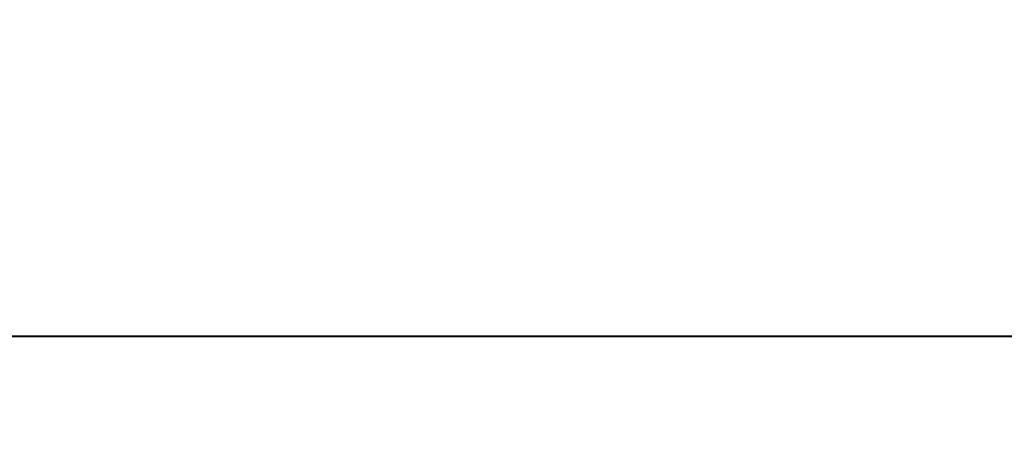
# Model space of a CAD drawing. Units: inches. Extents: x 459864 to 460310, y 324185 to 324787.
# Tile 81 of 112: x 460246.614 to 460247.1043, y 324283.4295 to 324283.6409. Entities that reach past the tile are written whole.
import ezdxf

# ---------------------------------------------------------------- set-up
doc = ezdxf.new("R2010")
doc.units = ezdxf.units.IN
for name, color, linetype, lineweight in [('A-ANNO-DIMS', 2, 'Continuous', 18), ('A-WALL', 7, 'Continuous', 40), ('L-SITE-PATT', 252, 'Continuous', 13)]:
    doc.layers.add(name, color=color, linetype=linetype, lineweight=lineweight)
doc.styles.get("Standard").update_dxf_attribs({"font": 'arial.ttf'})
doc.dimstyles.new('ISO-25', dxfattribs={"dimtxt": 6, "dimasz": 2.5, "dimexe": 1.25, "dimexo": 0.625, "dimtad": 1, "dimdec": 1, "dimlunit": 3, "dimtxsty": 'Standard', "dimcen": 2.5, "dimadec": 0, "dimazin": 0, "dimtfac": 1, "dimtdec": 1, "dimtmove": 0, "dimatfit": 3, "dimfxl": 1, "dimarcsym": 0})

# ---------------------------------------------------------------- blocks, each defined once
blk = doc.blocks.new('*D67')
at = {"layer": 'A-ANNO-DIMS', "color": 0, "lineweight": -2, "transparency": 16777216}
for p, q in [((460208.11493, 324284.10823), (460208.11493, 324315.13323)), ((460247.11493, 324284.10823), (460247.11493, 324315.13323)), ((460210.61493, 324313.88323), (460244.61493, 324313.88323))]:
    blk.add_line(p, q, dxfattribs=at)
at = {"layer": 'A-ANNO-DIMS', "color": 0, "transparency": 16777216}
for points in [[(460210.61493, 324314.2999), (460210.61493, 324313.46657), (460208.11493, 324313.88323)], [(460244.61493, 324314.2999), (460244.61493, 324313.46657), (460247.11493, 324313.88323)]]:
    blk.add_solid(points, dxfattribs=at)
at = {"layer": 'Defpoints', "color": 0, "transparency": 16777216}
for p in [(460247.11493, 324313.88323), (460208.11493, 324283.48323), (460247.11493, 324283.48323)]:
    blk.add_point(p, dxfattribs=at)
at = {"layer": 'A-ANNO-DIMS', "color": 0, "transparency": 16777216, "insert": (460227.61493, 324317.57372), "char_height": 6, "attachment_point": 5}
blk.add_mtext('3\'-3"', dxfattribs=at)

msp = doc.modelspace()

# ---------------------------------------------------------------- hatches: boundary and pattern name
at = {"layer": 'L-SITE-PATT'}
h = msp.add_hatch(dxfattribs=at)
h.set_pattern_fill('DOTS', color=256)
h.paths.add_polyline_path([(460269.80361, 324283.48323), (460247.11493, 324283.48323), (460121.92928, 324283.48323), (460121.92928, 324252.47302), (460117.42928, 324252.47302), (460110.12356, 324252.47302), (460110.12356, 324243.28654), (460080.82954, 324243.28654), (460080.82954, 324252.47302), (460061.11493, 324252.47302), (460061.11493, 324251.88242), (460077.9089, 324251.88242), (460077.9089, 324199.48323), (460080.82954, 324199.48323), (460080.82954, 324207.55322), (460110.12356, 324207.55322), (460110.12356, 324199.48323), (460110.81335, 324199.48323), (460262.11493, 324199.48323), (460269.80361, 324199.48323)], flags=17)
edge = h.paths.add_edge_path(flags=0)
edge.add_ellipse((460222.5903, 324263.81323), major_axis=(-8.48528, 8.48528), ratio=1, start_angle=405, end_angle=495, ccw=False)
edge.add_line((460214.82087, 324254.65989), (460214.83162, 324254.66592))
edge.add_ellipse((460222.5903, 324263.81323), major_axis=(-8.48528, 8.48528), ratio=1, start_angle=405, end_angle=495, ccw=False)
edge.add_line((460210.75891, 324261.78055), (460210.76758, 324261.78682))
edge.add_ellipse((460222.5903, 324263.81323), major_axis=(-8.48528, 8.48528), ratio=1, start_angle=405, end_angle=495, ccw=False)
edge.add_ellipse((460222.5903, 324263.81323), major_axis=(-8.48528, 8.48528), ratio=1, start_angle=392.754016, end_angle=405, ccw=False)
edge.add_ellipse((460222.5903, 324263.81323), major_axis=(-8.48528, 8.48528), ratio=1, start_angle=380.934718, end_angle=392.754016, ccw=False)
edge.add_line((460211.33706, 324267.98503), (460211.3404, 324267.98503))
edge.add_ellipse((460222.5903, 324263.81323), major_axis=(-8.48528, 8.48528), ratio=1, start_angle=380.934718, end_angle=392.754016, ccw=False)
edge.add_ellipse((460222.5903, 324263.81323), major_axis=(-8.48528, 8.48528), ratio=1, start_angle=347.901521, end_angle=380.934718, ccw=False)
edge.add_ellipse((460222.5903, 324263.81323), major_axis=(-8.48528, 8.48528), ratio=1, start_angle=327.061924, end_angle=347.901521, ccw=False)
edge.add_ellipse((460222.5903, 324263.81323), major_axis=(-8.48528, 8.48528), ratio=1, start_angle=278.324642, end_angle=327.061924, ccw=False)
edge.add_line((460225.15828, 324275.53599), (460225.1577, 324275.53464))
edge.add_ellipse((460222.5903, 324263.81323), major_axis=(-8.48528, 8.48528), ratio=1, start_angle=278.324642, end_angle=327.061924, ccw=False)
edge.add_ellipse((460222.5903, 324263.81323), major_axis=(-8.48528, 8.48528), ratio=1, start_angle=260.643569, end_angle=278.324642, ccw=False)
edge.add_ellipse((460222.5903, 324263.81323), major_axis=(-8.48528, 8.48528), ratio=1, start_angle=225, end_angle=260.643569, ccw=False)
edge.add_line((460234.50879, 324265.2428), (460234.50146, 324265.23944))
edge.add_ellipse((460222.5903, 324263.81323), major_axis=(-8.48528, 8.48528), ratio=1, start_angle=225, end_angle=260.643569, ccw=False)
edge.add_ellipse((460222.5903, 324263.81323), major_axis=(-8.48528, 8.48528), ratio=1, start_angle=495, end_angle=585, ccw=False)
edge.add_line((460234.43667, 324261.86121), (460234.42378, 324261.85782))
edge.add_ellipse((460222.5903, 324263.81323), major_axis=(-8.48528, 8.48528), ratio=1, start_angle=495, end_angle=585, ccw=False)
edge.add_line((460227.95013, 324253.06719), (460227.94641, 324253.08314))
edge.add_ellipse((460222.5903, 324263.81323), major_axis=(-8.48528, 8.48528), ratio=1, start_angle=495, end_angle=585, ccw=False)
edge.add_line((460226.22298, 324252.36927), (460226.21103, 324252.37955))
edge.add_ellipse((460222.5903, 324263.81323), major_axis=(-8.48528, 8.48528), ratio=1, start_angle=495, end_angle=585, ccw=False)
h.paths.add_polyline_path([(460219.65145, 324254.34665), (460218.46131, 324253.54498), (460218.27544, 324254.78932), (460219.6424, 324256.54177), (460219.62463, 324260.84756), (460216.11009, 324257.33302), (460214.34997, 324256.97807), (460215.41637, 324259.35568), (460212.52393, 324258.49582), (460213.13731, 324259.9298), (460218.50721, 324263.81323), (460222.5903, 324263.81323), (460222.5903, 324267.8067), (460218.17554, 324272.21231), (460219.02597, 324274.63898), (460222.5903, 324272.81113), (460222.5903, 324275.42332), (460223.0571, 324274.82493), (460222.67523, 324273.49221), (460225.91168, 324267.13461), (460219.62463, 324260.84756)], flags=0)
edge = h.paths.add_edge_path(flags=0)
edge.add_ellipse((460194.57576, 324264.04649), major_axis=(-8.48528, 8.48528), ratio=1, start_angle=495, end_angle=585, ccw=False)
edge.add_line((460199.93559, 324253.30046), (460199.93188, 324253.31641))
edge.add_ellipse((460194.57576, 324264.04649), major_axis=(-8.48528, 8.48528), ratio=1, start_angle=495, end_angle=585, ccw=False)
edge.add_line((460198.20844, 324252.60253), (460198.19649, 324252.61282))
edge.add_ellipse((460194.57576, 324264.04649), major_axis=(-8.48528, 8.48528), ratio=1, start_angle=495, end_angle=585, ccw=False)
edge.add_ellipse((460194.57576, 324264.04649), major_axis=(-8.48528, 8.48528), ratio=1, start_angle=405, end_angle=495, ccw=False)
edge.add_line((460186.80633, 324254.89316), (460186.81708, 324254.89919))
edge.add_ellipse((460194.57576, 324264.04649), major_axis=(-8.48528, 8.48528), ratio=1, start_angle=405, end_angle=495, ccw=False)
edge.add_line((460182.74437, 324262.01382), (460182.75305, 324262.02009))
edge.add_ellipse((460194.57576, 324264.04649), major_axis=(-8.48528, 8.48528), ratio=1, start_angle=405, end_angle=495, ccw=False)
edge.add_ellipse((460194.57576, 324264.04649), major_axis=(-8.48528, 8.48528), ratio=1, start_angle=392.754016, end_angle=405, ccw=False)
edge.add_ellipse((460194.57576, 324264.04649), major_axis=(-8.48528, 8.48528), ratio=1, start_angle=380.934718, end_angle=392.754016, ccw=False)
edge.add_line((460183.32252, 324268.21829), (460183.32587, 324268.21829))
edge.add_ellipse((460194.57576, 324264.04649), major_axis=(-8.48528, 8.48528), ratio=1, start_angle=380.934718, end_angle=392.754016, ccw=False)
edge.add_ellipse((460194.57576, 324264.04649), major_axis=(-8.48528, 8.48528), ratio=1, start_angle=347.901521, end_angle=380.934718, ccw=False)
edge.add_ellipse((460194.57576, 324264.04649), major_axis=(-8.48528, 8.48528), ratio=1, start_angle=327.061924, end_angle=347.901521, ccw=False)
edge.add_ellipse((460194.57576, 324264.04649), major_axis=(-8.48528, 8.48528), ratio=1, start_angle=278.324642, end_angle=327.061924, ccw=False)
edge.add_line((460197.14374, 324275.76926), (460197.14316, 324275.7679))
edge.add_ellipse((460194.57576, 324264.04649), major_axis=(-8.48528, 8.48528), ratio=1, start_angle=278.324642, end_angle=327.061924, ccw=False)
edge.add_ellipse((460194.57576, 324264.04649), major_axis=(-8.48528, 8.48528), ratio=1, start_angle=260.643569, end_angle=278.324642, ccw=False)
edge.add_ellipse((460194.57576, 324264.04649), major_axis=(-8.48528, 8.48528), ratio=1, start_angle=225, end_angle=260.643569, ccw=False)
edge.add_line((460206.49425, 324265.47606), (460206.48692, 324265.47271))
edge.add_ellipse((460194.57576, 324264.04649), major_axis=(-8.48528, 8.48528), ratio=1, start_angle=225, end_angle=260.643569, ccw=False)
edge.add_ellipse((460194.57576, 324264.04649), major_axis=(-8.48528, 8.48528), ratio=1, start_angle=495, end_angle=585, ccw=False)
edge.add_line((460206.42213, 324262.09448), (460206.40925, 324262.09109))
h.paths.add_polyline_path([(460191.61009, 324261.08083), (460191.63691, 324254.57992), (460190.44677, 324253.77825), (460190.2609, 324255.02259), (460191.62786, 324256.77503), (460191.61009, 324261.08083), (460188.09555, 324257.56629), (460186.33543, 324257.21133), (460187.40183, 324259.58894), (460184.5094, 324258.72909), (460185.12278, 324260.16306), (460190.49267, 324264.04649), (460194.57576, 324264.04649), (460194.57576, 324268.03996), (460190.161, 324272.44558), (460191.01143, 324274.87225), (460194.57576, 324273.04439), (460194.57576, 324275.65659), (460195.04256, 324275.0582), (460194.66069, 324273.72548), (460197.89714, 324267.36788)], flags=0)
edge = h.paths.add_edge_path(flags=0)
edge.add_ellipse((460252.91196, 324263.57762), major_axis=(-8.48528, 8.48528), ratio=1, start_angle=405, end_angle=495, ccw=False)
edge.add_line((460241.08058, 324261.54494), (460241.08925, 324261.55121))
edge.add_ellipse((460252.91196, 324263.57762), major_axis=(-8.48528, 8.48528), ratio=1, start_angle=405, end_angle=495, ccw=False)
edge.add_ellipse((460252.91196, 324263.57762), major_axis=(-8.48528, 8.48528), ratio=1, start_angle=392.754016, end_angle=405, ccw=False)
edge.add_ellipse((460252.91196, 324263.57762), major_axis=(-8.48528, 8.48528), ratio=1, start_angle=380.934718, end_angle=392.754016, ccw=False)
edge.add_line((460241.65872, 324267.74942), (460241.66207, 324267.74942))
edge.add_ellipse((460252.91196, 324263.57762), major_axis=(-8.48528, 8.48528), ratio=1, start_angle=380.934718, end_angle=392.754016, ccw=False)
edge.add_ellipse((460252.91196, 324263.57762), major_axis=(-8.48528, 8.48528), ratio=1, start_angle=347.901521, end_angle=380.934718, ccw=False)
edge.add_ellipse((460252.91196, 324263.57762), major_axis=(-8.48528, 8.48528), ratio=1, start_angle=327.061924, end_angle=347.901521, ccw=False)
edge.add_ellipse((460252.91196, 324263.57762), major_axis=(-8.48528, 8.48528), ratio=1, start_angle=278.324642, end_angle=327.061924, ccw=False)
edge.add_line((460255.47994, 324275.30038), (460255.47936, 324275.29902))
edge.add_ellipse((460252.91196, 324263.57762), major_axis=(-8.48528, 8.48528), ratio=1, start_angle=278.324642, end_angle=327.061924, ccw=False)
edge.add_ellipse((460252.91196, 324263.57762), major_axis=(-8.48528, 8.48528), ratio=1, start_angle=260.643569, end_angle=278.324642, ccw=False)
edge.add_ellipse((460252.91196, 324263.57762), major_axis=(-8.48528, 8.48528), ratio=1, start_angle=225, end_angle=260.643569, ccw=False)
edge.add_line((460264.83046, 324265.00718), (460264.82312, 324265.00383))
edge.add_ellipse((460252.91196, 324263.57762), major_axis=(-8.48528, 8.48528), ratio=1, start_angle=225, end_angle=260.643569, ccw=False)
edge.add_ellipse((460252.91196, 324263.57762), major_axis=(-8.48528, 8.48528), ratio=1, start_angle=495, end_angle=585, ccw=False)
edge.add_line((460264.75833, 324261.6256), (460264.74545, 324261.62221))
edge.add_ellipse((460252.91196, 324263.57762), major_axis=(-8.48528, 8.48528), ratio=1, start_angle=495, end_angle=585, ccw=False)
edge.add_line((460258.2718, 324252.83158), (460258.26808, 324252.84753))
edge.add_ellipse((460252.91196, 324263.57762), major_axis=(-8.48528, 8.48528), ratio=1, start_angle=495, end_angle=585, ccw=False)
edge.add_line((460256.54464, 324252.13365), (460256.5327, 324252.14394))
edge.add_ellipse((460252.91196, 324263.57762), major_axis=(-8.48528, 8.48528), ratio=1, start_angle=495, end_angle=585, ccw=False)
edge.add_ellipse((460252.91196, 324263.57762), major_axis=(-8.48528, 8.48528), ratio=1, start_angle=405, end_angle=495, ccw=False)
edge.add_line((460245.14253, 324254.42428), (460245.15329, 324254.43031))
h.paths.add_polyline_path([(460244.67163, 324256.74245), (460245.73803, 324259.12007), (460242.8456, 324258.26021), (460243.45898, 324259.69418), (460248.82888, 324263.57762), (460252.91196, 324263.57762), (460252.91196, 324267.57108), (460248.4972, 324271.9767), (460249.34763, 324274.40337), (460252.91196, 324272.57552), (460252.91196, 324275.18771), (460253.37876, 324274.58932), (460252.9969, 324273.2566), (460256.23334, 324266.899), (460249.9463, 324260.61195), (460249.97312, 324254.11104), (460248.78298, 324253.30937), (460248.5971, 324254.55371), (460249.96406, 324256.30615), (460249.9463, 324260.61195), (460246.43175, 324257.09741)], flags=0)
edge = h.paths.add_edge_path(flags=0)
edge.add_ellipse((460167.43869, 324262.83279), major_axis=(-8.48528, 8.48528), ratio=1, start_angle=495, end_angle=585, ccw=False)
edge.add_line((460172.79852, 324252.08676), (460172.79481, 324252.1027))
edge.add_ellipse((460167.43869, 324262.83279), major_axis=(-8.48528, 8.48528), ratio=1, start_angle=495, end_angle=585, ccw=False)
edge.add_line((460171.07137, 324251.38883), (460171.05942, 324251.39911))
edge.add_ellipse((460167.43869, 324262.83279), major_axis=(-8.48528, 8.48528), ratio=1, start_angle=495, end_angle=585, ccw=False)
edge.add_ellipse((460167.43869, 324262.83279), major_axis=(-8.48528, 8.48528), ratio=1, start_angle=405, end_angle=495, ccw=False)
edge.add_line((460159.66926, 324253.67945), (460159.68001, 324253.68548))
edge.add_ellipse((460167.43869, 324262.83279), major_axis=(-8.48528, 8.48528), ratio=1, start_angle=405, end_angle=495, ccw=False)
edge.add_line((460155.6073, 324260.80011), (460155.61598, 324260.80639))
edge.add_ellipse((460167.43869, 324262.83279), major_axis=(-8.48528, 8.48528), ratio=1, start_angle=405, end_angle=495, ccw=False)
edge.add_ellipse((460167.43869, 324262.83279), major_axis=(-8.48528, 8.48528), ratio=1, start_angle=392.754016, end_angle=405, ccw=False)
edge.add_ellipse((460167.43869, 324262.83279), major_axis=(-8.48528, 8.48528), ratio=1, start_angle=380.934718, end_angle=392.754016, ccw=False)
edge.add_line((460156.18545, 324267.00459), (460156.1888, 324267.00459))
edge.add_ellipse((460167.43869, 324262.83279), major_axis=(-8.48528, 8.48528), ratio=1, start_angle=380.934718, end_angle=392.754016, ccw=False)
edge.add_ellipse((460167.43869, 324262.83279), major_axis=(-8.48528, 8.48528), ratio=1, start_angle=347.901521, end_angle=380.934718, ccw=False)
edge.add_ellipse((460167.43869, 324262.83279), major_axis=(-8.48528, 8.48528), ratio=1, start_angle=327.061924, end_angle=347.901521, ccw=False)
edge.add_ellipse((460167.43869, 324262.83279), major_axis=(-8.48528, 8.48528), ratio=1, start_angle=278.324642, end_angle=327.061924, ccw=False)
edge.add_line((460170.00667, 324274.55555), (460170.00609, 324274.5542))
edge.add_ellipse((460167.43869, 324262.83279), major_axis=(-8.48528, 8.48528), ratio=1, start_angle=278.324642, end_angle=327.061924, ccw=False)
edge.add_ellipse((460167.43869, 324262.83279), major_axis=(-8.48528, 8.48528), ratio=1, start_angle=260.643569, end_angle=278.324642, ccw=False)
edge.add_ellipse((460167.43869, 324262.83279), major_axis=(-8.48528, 8.48528), ratio=1, start_angle=225, end_angle=260.643569, ccw=False)
edge.add_line((460179.35719, 324264.26236), (460179.34985, 324264.259))
edge.add_ellipse((460167.43869, 324262.83279), major_axis=(-8.48528, 8.48528), ratio=1, start_angle=225, end_angle=260.643569, ccw=False)
edge.add_ellipse((460167.43869, 324262.83279), major_axis=(-8.48528, 8.48528), ratio=1, start_angle=495, end_angle=585, ccw=False)
edge.add_line((460179.28506, 324260.88078), (460179.27218, 324260.87738))
h.paths.add_polyline_path([(460164.47302, 324259.86713), (460164.49985, 324253.36622), (460163.30971, 324252.56455), (460163.12383, 324253.80888), (460164.49079, 324255.56133), (460164.47302, 324259.86713), (460160.95848, 324256.35258), (460159.19836, 324255.99763), (460160.26476, 324258.37524), (460157.37233, 324257.51539), (460157.98571, 324258.94936), (460163.35561, 324262.83279), (460167.43869, 324262.83279), (460167.43869, 324266.82626), (460163.02393, 324271.23187), (460163.87436, 324273.65854), (460167.43869, 324271.83069), (460167.43869, 324274.44288), (460167.90549, 324273.84449), (460167.52362, 324272.51177), (460170.76007, 324266.15417)], flags=0)
edge = h.paths.add_edge_path(flags=0)
edge.add_ellipse((460140.75809, 324262.36958), major_axis=(-8.48528, 8.48528), ratio=1, start_angle=495, end_angle=585, ccw=False)
edge.add_line((460146.11792, 324251.62355), (460146.11421, 324251.6395))
edge.add_ellipse((460140.75809, 324262.36958), major_axis=(-8.48528, 8.48528), ratio=1, start_angle=495, end_angle=585, ccw=False)
edge.add_line((460144.39077, 324250.92562), (460144.37882, 324250.93591))
edge.add_ellipse((460140.75809, 324262.36958), major_axis=(-8.48528, 8.48528), ratio=1, start_angle=495, end_angle=585, ccw=False)
edge.add_ellipse((460140.75809, 324262.36958), major_axis=(-8.48528, 8.48528), ratio=1, start_angle=405, end_angle=495, ccw=False)
edge.add_line((460132.98866, 324253.21625), (460132.99941, 324253.22228))
edge.add_ellipse((460140.75809, 324262.36958), major_axis=(-8.48528, 8.48528), ratio=1, start_angle=405, end_angle=495, ccw=False)
edge.add_line((460128.9267, 324260.33691), (460128.93538, 324260.34318))
edge.add_ellipse((460140.75809, 324262.36958), major_axis=(-8.48528, 8.48528), ratio=1, start_angle=405, end_angle=495, ccw=False)
edge.add_ellipse((460140.75809, 324262.36958), major_axis=(-8.48528, 8.48528), ratio=1, start_angle=392.754016, end_angle=405, ccw=False)
edge.add_ellipse((460140.75809, 324262.36958), major_axis=(-8.48528, 8.48528), ratio=1, start_angle=380.934718, end_angle=392.754016, ccw=False)
edge.add_line((460129.50485, 324266.54138), (460129.5082, 324266.54138))
edge.add_ellipse((460140.75809, 324262.36958), major_axis=(-8.48528, 8.48528), ratio=1, start_angle=380.934718, end_angle=392.754016, ccw=False)
edge.add_ellipse((460140.75809, 324262.36958), major_axis=(-8.48528, 8.48528), ratio=1, start_angle=347.901521, end_angle=380.934718, ccw=False)
edge.add_ellipse((460140.75809, 324262.36958), major_axis=(-8.48528, 8.48528), ratio=1, start_angle=327.061924, end_angle=347.901521, ccw=False)
edge.add_ellipse((460140.75809, 324262.36958), major_axis=(-8.48528, 8.48528), ratio=1, start_angle=278.324642, end_angle=327.061924, ccw=False)
edge.add_line((460143.32607, 324274.09235), (460143.32549, 324274.09099))
edge.add_ellipse((460140.75809, 324262.36958), major_axis=(-8.48528, 8.48528), ratio=1, start_angle=278.324642, end_angle=327.061924, ccw=False)
edge.add_ellipse((460140.75809, 324262.36958), major_axis=(-8.48528, 8.48528), ratio=1, start_angle=260.643569, end_angle=278.324642, ccw=False)
edge.add_ellipse((460140.75809, 324262.36958), major_axis=(-8.48528, 8.48528), ratio=1, start_angle=225, end_angle=260.643569, ccw=False)
edge.add_line((460152.67658, 324263.79915), (460152.66925, 324263.7958))
edge.add_ellipse((460140.75809, 324262.36958), major_axis=(-8.48528, 8.48528), ratio=1, start_angle=225, end_angle=260.643569, ccw=False)
edge.add_ellipse((460140.75809, 324262.36958), major_axis=(-8.48528, 8.48528), ratio=1, start_angle=495, end_angle=585, ccw=False)
edge.add_line((460152.60446, 324260.41757), (460152.59158, 324260.41418))
h.paths.add_polyline_path([(460137.79242, 324259.40392), (460137.81925, 324252.90301), (460136.6291, 324252.10134), (460136.44323, 324253.34568), (460137.81019, 324255.09812), (460137.79242, 324259.40392), (460134.27788, 324255.88938), (460132.51776, 324255.53442), (460133.58416, 324257.91203), (460130.69173, 324257.05218), (460131.30511, 324258.48615), (460136.675, 324262.36958), (460140.75809, 324262.36958), (460140.75809, 324266.36305), (460136.34333, 324270.76867), (460137.19376, 324273.19534), (460140.75809, 324271.36749), (460140.75809, 324273.97968), (460141.22489, 324273.38129), (460140.84302, 324272.04857), (460144.07947, 324265.69097)], flags=0)
h.paths.add_polyline_path([(460110.12356, 324227.41387), (460080.82954, 324227.41387), (460080.82954, 324235.48385), (460110.12356, 324235.48385)], flags=16)
h.paths.add_polyline_path([(460110.12356, 324220.79663), (460110.12356, 324212.72665), (460080.82954, 324212.72665), (460080.82954, 324220.79663)], flags=16)
h.paths.add_polyline_path([(460269.80361, 324283.48323), (460247.11493, 324283.48323), (460121.92928, 324283.48323), (460121.92928, 324252.47302), (460117.42928, 324252.47302), (460110.12356, 324252.47302), (460110.12356, 324243.28654), (460080.82954, 324243.28654), (460080.82954, 324252.47302), (460061.11493, 324252.47302), (460061.11493, 324251.88242), (460077.9089, 324251.88242), (460077.9089, 324199.48323), (460080.82954, 324199.48323), (460080.82954, 324207.55322), (460110.12356, 324207.55322), (460110.12356, 324199.48323), (460262.11493, 324199.48323), (460269.80361, 324199.48323)], flags=17)
h.paths.add_polyline_path([(460219.65145, 324254.34665), (460218.46131, 324253.54498), (460218.27544, 324254.78932), (460219.6424, 324256.54177), (460219.62463, 324260.84756), (460216.11009, 324257.33302), (460214.34997, 324256.97807), (460215.41637, 324259.35568), (460212.52393, 324258.49582), (460213.13731, 324259.9298), (460218.50721, 324263.81323), (460222.5903, 324263.81323), (460220.18049, 324266.22304), (460215.46096, 324265.30765), (460211.83453, 324266.13655), (460216.24662, 324267.98503), (460218.4185, 324267.98503), (460222.5903, 324263.81323), (460222.5903, 324267.8067), (460218.17554, 324272.21231), (460219.02597, 324274.63898), (460222.5903, 324272.81113), (460222.5903, 324275.42332), (460223.0571, 324274.82493), (460222.67523, 324273.49221), (460225.91168, 324267.13461), (460222.5903, 324263.81323), (460231.38287, 324263.81323), (460228.48472, 324262.48783), (460224.42521, 324261.97832), (460228.6799, 324257.72362), (460228.96584, 324254.79101), (460227.14177, 324256.53663), (460227.54207, 324254.81857), (460227.33334, 324253.61447), (460222.5903, 324259.98463), (460222.5903, 324255.49667), (460221.37741, 324256.54085), (460220.57579, 324261.79873), (460219.62463, 324260.84756)], flags=0)
h.paths.add_polyline_path([(460199.12723, 324256.7699), (460199.52753, 324255.05184), (460199.31881, 324253.84773), (460194.57576, 324260.21789), (460194.57576, 324255.72993), (460193.36287, 324256.77411), (460192.56126, 324262.03199), (460191.61009, 324261.08083), (460191.63691, 324254.57992), (460190.44677, 324253.77825), (460190.2609, 324255.02259), (460191.62786, 324256.77503), (460191.61009, 324261.08083), (460188.09555, 324257.56629), (460186.33543, 324257.21133), (460187.40183, 324259.58894), (460184.5094, 324258.72909), (460185.12278, 324260.16306), (460190.49267, 324264.04649), (460194.57576, 324264.04649), (460192.16595, 324266.4563), (460187.44642, 324265.54091), (460183.82, 324266.36982), (460188.23208, 324268.21829), (460190.40396, 324268.21829), (460194.57576, 324264.04649), (460194.57576, 324268.03996), (460190.161, 324272.44558), (460191.01143, 324274.87225), (460194.57576, 324273.04439), (460194.57576, 324275.65659), (460195.04256, 324275.0582), (460194.66069, 324273.72548), (460197.89714, 324267.36788), (460194.57576, 324264.04649), (460203.36833, 324264.04649), (460200.47018, 324262.72109), (460196.41067, 324262.21158), (460200.66536, 324257.95689), (460200.9513, 324255.02428)], flags=0)
h.paths.add_polyline_path([(460244.67163, 324256.74245), (460245.73803, 324259.12007), (460242.8456, 324258.26021), (460243.45898, 324259.69418), (460248.82888, 324263.57762), (460252.91196, 324263.57762), (460250.50215, 324265.98742), (460245.78262, 324265.07203), (460242.1562, 324265.90094), (460246.56828, 324267.74942), (460248.74016, 324267.74942), (460252.91196, 324263.57762), (460252.91196, 324267.57108), (460248.4972, 324271.9767), (460249.34763, 324274.40337), (460252.91196, 324272.57552), (460252.91196, 324275.18771), (460253.37876, 324274.58932), (460252.9969, 324273.2566), (460256.23334, 324266.899), (460252.91196, 324263.57762), (460261.70454, 324263.57762), (460258.80638, 324262.25221), (460254.74687, 324261.7427), (460259.00157, 324257.48801), (460259.2875, 324254.5554), (460257.46343, 324256.30102), (460257.86373, 324254.58296), (460257.65501, 324253.37885), (460252.91196, 324259.74901), (460252.91196, 324255.26105), (460251.69907, 324256.30524), (460250.89746, 324261.56311), (460249.9463, 324260.61195), (460249.97312, 324254.11104), (460248.78298, 324253.30937), (460248.5971, 324254.55371), (460249.96406, 324256.30615), (460249.9463, 324260.61195), (460246.43175, 324257.09741)], flags=0)
h.paths.add_polyline_path([(460173.52829, 324256.74319), (460173.81423, 324253.81058), (460171.99016, 324255.55619), (460172.39046, 324253.83814), (460172.18174, 324252.63403), (460167.43869, 324259.00419), (460167.43869, 324254.51623), (460166.2258, 324255.56041), (460165.42419, 324260.81829), (460164.47302, 324259.86713), (460164.49985, 324253.36622), (460163.30971, 324252.56455), (460163.12383, 324253.80888), (460164.49079, 324255.56133), (460164.47302, 324259.86713), (460160.95848, 324256.35258), (460159.19836, 324255.99763), (460160.26476, 324258.37524), (460157.37233, 324257.51539), (460157.98571, 324258.94936), (460163.35561, 324262.83279), (460167.43869, 324262.83279), (460165.02888, 324265.2426), (460160.30935, 324264.32721), (460156.68293, 324265.15611), (460161.09501, 324267.00459), (460163.26689, 324267.00459), (460167.43869, 324262.83279), (460167.43869, 324266.82626), (460163.02393, 324271.23187), (460163.87436, 324273.65854), (460167.43869, 324271.83069), (460167.43869, 324274.44288), (460167.90549, 324273.84449), (460167.52362, 324272.51177), (460170.76007, 324266.15417), (460167.43869, 324262.83279), (460176.23127, 324262.83279), (460173.33311, 324261.50739), (460169.2736, 324260.99788)], flags=0)
h.paths.add_polyline_path([(460146.84769, 324256.27998), (460147.13363, 324253.34737), (460145.30956, 324255.09299), (460145.70986, 324253.37493), (460145.50114, 324252.17082), (460140.75809, 324258.54098), (460140.75809, 324254.05302), (460139.5452, 324255.0972), (460138.74359, 324260.35508), (460137.79242, 324259.40392), (460137.81925, 324252.90301), (460136.6291, 324252.10134), (460136.44323, 324253.34568), (460137.81019, 324255.09812), (460137.79242, 324259.40392), (460134.27788, 324255.88938), (460132.51776, 324255.53442), (460133.58416, 324257.91203), (460130.69173, 324257.05218), (460131.30511, 324258.48615), (460136.675, 324262.36958), (460140.75809, 324262.36958), (460138.34828, 324264.77939), (460133.62875, 324263.864), (460130.00233, 324264.69291), (460134.41441, 324266.54138), (460136.58629, 324266.54138), (460140.75809, 324262.36958), (460140.75809, 324266.36305), (460136.34333, 324270.76867), (460137.19376, 324273.19534), (460140.75809, 324271.36749), (460140.75809, 324273.97968), (460141.22489, 324273.38129), (460140.84302, 324272.04857), (460144.07947, 324265.69097), (460140.75809, 324262.36958), (460149.55066, 324262.36958), (460146.65251, 324261.04418), (460142.593, 324260.53467)], flags=0)
edge = h.paths.add_edge_path()
edge.add_line((460269.80361, 324272.54905), (460260.88148, 324272.54905))
edge.add_ellipse((460252.91196, 324263.57762), major_axis=(-8.48528, 8.48528), ratio=1, start_angle=260.643569, end_angle=273.384624, ccw=False)
edge.add_line((460262.28261, 324271.09211), (460262.26055, 324271.09106))
edge.add_ellipse((460252.91196, 324263.57762), major_axis=(-8.48528, 8.48528), ratio=1, start_angle=260.643569, end_angle=273.384624, ccw=False)
edge.add_ellipse((460252.91196, 324263.57762), major_axis=(-8.48528, 8.48528), ratio=1, start_angle=225, end_angle=260.643569, ccw=False)
edge.add_line((460263.60857, 324269.06329), (460263.57165, 324269.05828))
edge.add_ellipse((460252.91196, 324263.57762), major_axis=(-8.48528, 8.48528), ratio=1, start_angle=225, end_angle=260.643569, ccw=False)
edge.add_line((460264.61546, 324266.30554), (460264.58536, 324266.3052))
edge.add_ellipse((460252.91196, 324263.57762), major_axis=(-8.48528, 8.48528), ratio=1, start_angle=225, end_angle=260.643569, ccw=False)
edge.add_line((460264.83046, 324265.00718), (460264.82312, 324265.00383))
edge.add_ellipse((460252.91196, 324263.57762), major_axis=(-8.48528, 8.48528), ratio=1, start_angle=225, end_angle=260.643569, ccw=False)
edge.add_ellipse((460252.91196, 324263.57762), major_axis=(-8.48528, 8.48528), ratio=1, start_angle=495, end_angle=585, ccw=False)
edge.add_line((460264.75833, 324261.6256), (460264.74545, 324261.62221))
edge.add_ellipse((460252.91196, 324263.57762), major_axis=(-8.48528, 8.48528), ratio=1, start_angle=495, end_angle=585, ccw=False)
edge.add_line((460263.4422, 324257.73902), (460263.38926, 324257.77924))
edge.add_ellipse((460252.91196, 324263.57762), major_axis=(-8.48528, 8.48528), ratio=1, start_angle=495, end_angle=585, ccw=False)
edge.add_line((460258.12807, 324252.7435), (460258.10188, 324252.77868))
edge.add_ellipse((460252.91196, 324263.57762), major_axis=(-8.48528, 8.48528), ratio=1, start_angle=495, end_angle=585, ccw=False)
edge.add_line((460256.54464, 324252.13365), (460256.5327, 324252.14394))
edge.add_ellipse((460252.91196, 324263.57762), major_axis=(-8.48528, 8.48528), ratio=1, start_angle=495, end_angle=585, ccw=False)
edge.add_ellipse((460252.91196, 324263.57762), major_axis=(-8.48528, 8.48528), ratio=1, start_angle=405, end_angle=495, ccw=False)
edge.add_line((460250.59399, 324251.78041), (460250.60465, 324251.81982))
edge.add_ellipse((460252.91196, 324263.57762), major_axis=(-8.48528, 8.48528), ratio=1, start_angle=405, end_angle=495, ccw=False)
edge.add_line((460245.14253, 324254.42428), (460245.15329, 324254.43031))
edge.add_ellipse((460252.91196, 324263.57762), major_axis=(-8.48528, 8.48528), ratio=1, start_angle=405, end_angle=495, ccw=False)
edge.add_line((460243.52459, 324256.059), (460243.56034, 324256.09136))
edge.add_ellipse((460252.91196, 324263.57762), major_axis=(-8.48528, 8.48528), ratio=1, start_angle=405, end_angle=495, ccw=False)
edge.add_line((460241.4401, 324259.89273), (460241.52244, 324259.89588))
edge.add_ellipse((460252.91196, 324263.57762), major_axis=(-8.48528, 8.48528), ratio=1, start_angle=405, end_angle=495, ccw=False)
edge.add_line((460241.08058, 324261.54494), (460241.08925, 324261.55121))
edge.add_ellipse((460252.91196, 324263.57762), major_axis=(-8.48528, 8.48528), ratio=1, start_angle=405, end_angle=495, ccw=False)
edge.add_ellipse((460252.91196, 324263.57762), major_axis=(-8.48528, 8.48528), ratio=1, start_angle=392.754016, end_angle=405, ccw=False)
edge.add_line((460241.0503, 324265.43761), (460241.06257, 324265.44275))
edge.add_ellipse((460252.91196, 324263.57762), major_axis=(-8.48528, 8.48528), ratio=1, start_angle=392.754016, end_angle=405, ccw=False)
edge.add_ellipse((460252.91196, 324263.57762), major_axis=(-8.48528, 8.48528), ratio=1, start_angle=380.934718, end_angle=392.754016, ccw=False)
edge.add_line((460241.45189, 324267.17639), (460241.46904, 324267.17099))
edge.add_ellipse((460252.91196, 324263.57762), major_axis=(-8.48528, 8.48528), ratio=1, start_angle=380.934718, end_angle=392.754016, ccw=False)
edge.add_line((460241.65872, 324267.74942), (460241.66207, 324267.74942))
edge.add_ellipse((460252.91196, 324263.57762), major_axis=(-8.48528, 8.48528), ratio=1, start_angle=380.934718, end_angle=392.754016, ccw=False)
edge.add_ellipse((460252.91196, 324263.57762), major_axis=(-8.48528, 8.48528), ratio=1, start_angle=356.615376, end_angle=380.934718, ccw=False)
edge.add_line((460244.88029, 324272.48765), (460244.71265, 324272.54905))
edge.add_line((460244.71265, 324272.54905), (460230.81741, 324272.54905))
edge.add_ellipse((460222.5903, 324263.81323), major_axis=(-8.48528, 8.48528), ratio=1, start_angle=260.643569, end_angle=271.717775, ccw=False)
edge.add_ellipse((460222.5903, 324263.81323), major_axis=(-8.48528, 8.48528), ratio=1, start_angle=225, end_angle=260.643569, ccw=False)
edge.add_line((460233.2869, 324269.29891), (460233.24999, 324269.2939))
edge.add_ellipse((460222.5903, 324263.81323), major_axis=(-8.48528, 8.48528), ratio=1, start_angle=225, end_angle=260.643569, ccw=False)
edge.add_line((460234.2938, 324266.54115), (460234.26369, 324266.54081))
edge.add_ellipse((460222.5903, 324263.81323), major_axis=(-8.48528, 8.48528), ratio=1, start_angle=225, end_angle=260.643569, ccw=False)
edge.add_line((460234.50879, 324265.2428), (460234.50146, 324265.23944))
edge.add_ellipse((460222.5903, 324263.81323), major_axis=(-8.48528, 8.48528), ratio=1, start_angle=225, end_angle=260.643569, ccw=False)
edge.add_ellipse((460222.5903, 324263.81323), major_axis=(-8.48528, 8.48528), ratio=1, start_angle=495, end_angle=585, ccw=False)
edge.add_line((460234.43667, 324261.86121), (460234.42378, 324261.85782))
edge.add_ellipse((460222.5903, 324263.81323), major_axis=(-8.48528, 8.48528), ratio=1, start_angle=495, end_angle=585, ccw=False)
edge.add_line((460233.12054, 324257.97463), (460233.06759, 324258.01485))
edge.add_ellipse((460222.5903, 324263.81323), major_axis=(-8.48528, 8.48528), ratio=1, start_angle=495, end_angle=585, ccw=False)
edge.add_line((460227.8064, 324252.97912), (460227.78021, 324253.0143))
edge.add_ellipse((460222.5903, 324263.81323), major_axis=(-8.48528, 8.48528), ratio=1, start_angle=495, end_angle=585, ccw=False)
edge.add_line((460226.22298, 324252.36927), (460226.21103, 324252.37955))
edge.add_ellipse((460222.5903, 324263.81323), major_axis=(-8.48528, 8.48528), ratio=1, start_angle=495, end_angle=585, ccw=False)
edge.add_ellipse((460222.5903, 324263.81323), major_axis=(-8.48528, 8.48528), ratio=1, start_angle=405, end_angle=495, ccw=False)
edge.add_line((460220.27232, 324252.01602), (460220.28299, 324252.05543))
edge.add_ellipse((460222.5903, 324263.81323), major_axis=(-8.48528, 8.48528), ratio=1, start_angle=405, end_angle=495, ccw=False)
edge.add_line((460214.82087, 324254.65989), (460214.83162, 324254.66592))
edge.add_ellipse((460222.5903, 324263.81323), major_axis=(-8.48528, 8.48528), ratio=1, start_angle=405, end_angle=495, ccw=False)
edge.add_line((460213.20292, 324256.29462), (460213.23868, 324256.32697))
edge.add_ellipse((460222.5903, 324263.81323), major_axis=(-8.48528, 8.48528), ratio=1, start_angle=405, end_angle=495, ccw=False)
edge.add_line((460211.11844, 324260.12834), (460211.20077, 324260.13149))
edge.add_ellipse((460222.5903, 324263.81323), major_axis=(-8.48528, 8.48528), ratio=1, start_angle=405, end_angle=495, ccw=False)
edge.add_line((460210.75891, 324261.78055), (460210.76758, 324261.78682))
edge.add_ellipse((460222.5903, 324263.81323), major_axis=(-8.48528, 8.48528), ratio=1, start_angle=405, end_angle=495, ccw=False)
edge.add_ellipse((460222.5903, 324263.81323), major_axis=(-8.48528, 8.48528), ratio=1, start_angle=392.754016, end_angle=405, ccw=False)
edge.add_line((460210.72863, 324265.67323), (460210.7409, 324265.67836))
edge.add_ellipse((460222.5903, 324263.81323), major_axis=(-8.48528, 8.48528), ratio=1, start_angle=392.754016, end_angle=405, ccw=False)
edge.add_ellipse((460222.5903, 324263.81323), major_axis=(-8.48528, 8.48528), ratio=1, start_angle=380.934718, end_angle=392.754016, ccw=False)
edge.add_line((460211.13022, 324267.412), (460211.14738, 324267.4066))
edge.add_ellipse((460222.5903, 324263.81323), major_axis=(-8.48528, 8.48528), ratio=1, start_angle=380.934718, end_angle=392.754016, ccw=False)
edge.add_line((460211.33706, 324267.98503), (460211.3404, 324267.98503))
edge.add_ellipse((460222.5903, 324263.81323), major_axis=(-8.48528, 8.48528), ratio=1, start_angle=380.934718, end_angle=392.754016, ccw=False)
edge.add_ellipse((460222.5903, 324263.81323), major_axis=(-8.48528, 8.48528), ratio=1, start_angle=358.282225, end_angle=380.934718, ccw=False)
edge.add_line((460213.70452, 324271.90183), (460213.70904, 324271.86897))
edge.add_ellipse((460222.5903, 324263.81323), major_axis=(-8.48528, 8.48528), ratio=1, start_angle=358.282225, end_angle=380.934718, ccw=False)
edge.add_line((460214.36318, 324272.54905), (460203.07832, 324272.54905))
edge.add_line((460203.07832, 324272.54905), (460203.06034, 324272.53108))
edge.add_ellipse((460194.57576, 324264.04649), major_axis=(-8.48528, 8.48528), ratio=1, start_angle=260.643569, end_angle=270.11679, ccw=False)
edge.add_line((460203.95659, 324271.56147), (460203.92091, 324271.55978))
edge.add_ellipse((460194.57576, 324264.04649), major_axis=(-8.48528, 8.48528), ratio=1, start_angle=260.643569, end_angle=270.11679, ccw=False)
edge.add_ellipse((460194.57576, 324264.04649), major_axis=(-8.48528, 8.48528), ratio=1, start_angle=225, end_angle=260.643569, ccw=False)
edge.add_line((460205.27237, 324269.53217), (460205.23545, 324269.52716))
edge.add_ellipse((460194.57576, 324264.04649), major_axis=(-8.48528, 8.48528), ratio=1, start_angle=225, end_angle=260.643569, ccw=False)
edge.add_line((460206.27926, 324266.77442), (460206.24915, 324266.77407))
edge.add_ellipse((460194.57576, 324264.04649), major_axis=(-8.48528, 8.48528), ratio=1, start_angle=225, end_angle=260.643569, ccw=False)
edge.add_line((460206.49425, 324265.47606), (460206.48692, 324265.47271))
edge.add_ellipse((460194.57576, 324264.04649), major_axis=(-8.48528, 8.48528), ratio=1, start_angle=225, end_angle=260.643569, ccw=False)
edge.add_ellipse((460194.57576, 324264.04649), major_axis=(-8.48528, 8.48528), ratio=1, start_angle=495, end_angle=585, ccw=False)
edge.add_line((460206.42213, 324262.09448), (460206.40925, 324262.09109))
edge.add_ellipse((460194.57576, 324264.04649), major_axis=(-8.48528, 8.48528), ratio=1, start_angle=495, end_angle=585, ccw=False)
edge.add_line((460205.106, 324258.2079), (460205.05306, 324258.24812))
edge.add_ellipse((460194.57576, 324264.04649), major_axis=(-8.48528, 8.48528), ratio=1, start_angle=495, end_angle=585, ccw=False)
edge.add_line((460199.79187, 324253.21238), (460199.76568, 324253.24756))
edge.add_ellipse((460194.57576, 324264.04649), major_axis=(-8.48528, 8.48528), ratio=1, start_angle=495, end_angle=585, ccw=False)
edge.add_line((460198.20844, 324252.60253), (460198.19649, 324252.61282))
edge.add_ellipse((460194.57576, 324264.04649), major_axis=(-8.48528, 8.48528), ratio=1, start_angle=495, end_angle=585, ccw=False)
edge.add_ellipse((460194.57576, 324264.04649), major_axis=(-8.48528, 8.48528), ratio=1, start_angle=405, end_angle=495, ccw=False)
edge.add_line((460192.25779, 324252.24929), (460192.26845, 324252.2887))
edge.add_ellipse((460194.57576, 324264.04649), major_axis=(-8.48528, 8.48528), ratio=1, start_angle=405, end_angle=495, ccw=False)
edge.add_line((460186.80633, 324254.89316), (460186.81708, 324254.89919))
edge.add_ellipse((460194.57576, 324264.04649), major_axis=(-8.48528, 8.48528), ratio=1, start_angle=405, end_angle=495, ccw=False)
edge.add_line((460185.18839, 324256.52788), (460185.22414, 324256.56024))
edge.add_ellipse((460194.57576, 324264.04649), major_axis=(-8.48528, 8.48528), ratio=1, start_angle=405, end_angle=495, ccw=False)
edge.add_line((460183.1039, 324260.3616), (460183.18624, 324260.36476))
edge.add_ellipse((460194.57576, 324264.04649), major_axis=(-8.48528, 8.48528), ratio=1, start_angle=405, end_angle=495, ccw=False)
edge.add_line((460182.74437, 324262.01382), (460182.75305, 324262.02009))
edge.add_ellipse((460194.57576, 324264.04649), major_axis=(-8.48528, 8.48528), ratio=1, start_angle=405, end_angle=495, ccw=False)
edge.add_ellipse((460194.57576, 324264.04649), major_axis=(-8.48528, 8.48528), ratio=1, start_angle=392.754016, end_angle=405, ccw=False)
edge.add_line((460182.7141, 324265.90649), (460182.72636, 324265.91163))
edge.add_ellipse((460194.57576, 324264.04649), major_axis=(-8.48528, 8.48528), ratio=1, start_angle=392.754016, end_angle=405, ccw=False)
edge.add_ellipse((460194.57576, 324264.04649), major_axis=(-8.48528, 8.48528), ratio=1, start_angle=380.934718, end_angle=392.754016, ccw=False)
edge.add_line((460183.11568, 324267.64527), (460183.13284, 324267.63987))
edge.add_ellipse((460194.57576, 324264.04649), major_axis=(-8.48528, 8.48528), ratio=1, start_angle=380.934718, end_angle=392.754016, ccw=False)
edge.add_line((460183.32252, 324268.21829), (460183.32587, 324268.21829))
edge.add_ellipse((460194.57576, 324264.04649), major_axis=(-8.48528, 8.48528), ratio=1, start_angle=380.934718, end_angle=392.754016, ccw=False)
edge.add_ellipse((460194.57576, 324264.04649), major_axis=(-8.48528, 8.48528), ratio=1, start_angle=359.88321, end_angle=380.934718, ccw=False)
edge.add_line((460184.49136, 324270.61077), (460184.55315, 324270.61077))
edge.add_ellipse((460194.57576, 324264.04649), major_axis=(-8.48528, 8.48528), ratio=1, start_angle=359.88321, end_angle=380.934718, ccw=False)
edge.add_line((460185.34584, 324271.76024), (460185.37863, 324271.72802))
edge.add_ellipse((460194.57576, 324264.04649), major_axis=(-8.48528, 8.48528), ratio=1, start_angle=359.88321, end_angle=380.934718, ccw=False)
edge.add_line((460185.69672, 324272.08618), (460185.633, 324272.54905))
edge.add_line((460185.633, 324272.54905), (460174.68345, 324272.54905))
edge.add_line((460174.68345, 324272.54905), (460174.60605, 324272.45718))
edge.add_ellipse((460167.43869, 324262.83279), major_axis=(-8.48528, 8.48528), ratio=1, start_angle=260.643569, end_angle=278.324642, ccw=False)
edge.add_ellipse((460167.43869, 324262.83279), major_axis=(-8.48528, 8.48528), ratio=1, start_angle=225, end_angle=260.643569, ccw=False)
edge.add_line((460178.1353, 324268.31847), (460178.09838, 324268.31346))
edge.add_ellipse((460167.43869, 324262.83279), major_axis=(-8.48528, 8.48528), ratio=1, start_angle=225, end_angle=260.643569, ccw=False)
edge.add_line((460179.14219, 324265.56072), (460179.11209, 324265.56037))
edge.add_ellipse((460167.43869, 324262.83279), major_axis=(-8.48528, 8.48528), ratio=1, start_angle=225, end_angle=260.643569, ccw=False)
edge.add_line((460179.35719, 324264.26236), (460179.34985, 324264.259))
edge.add_ellipse((460167.43869, 324262.83279), major_axis=(-8.48528, 8.48528), ratio=1, start_angle=225, end_angle=260.643569, ccw=False)
edge.add_ellipse((460167.43869, 324262.83279), major_axis=(-8.48528, 8.48528), ratio=1, start_angle=495, end_angle=585, ccw=False)
edge.add_line((460179.28506, 324260.88078), (460179.27218, 324260.87738))
edge.add_ellipse((460167.43869, 324262.83279), major_axis=(-8.48528, 8.48528), ratio=1, start_angle=495, end_angle=585, ccw=False)
edge.add_line((460177.96893, 324256.99419), (460177.91599, 324257.03442))
edge.add_ellipse((460167.43869, 324262.83279), major_axis=(-8.48528, 8.48528), ratio=1, start_angle=495, end_angle=585, ccw=False)
edge.add_line((460172.6548, 324251.99868), (460172.62861, 324252.03386))
edge.add_ellipse((460167.43869, 324262.83279), major_axis=(-8.48528, 8.48528), ratio=1, start_angle=495, end_angle=585, ccw=False)
edge.add_line((460171.07137, 324251.38883), (460171.05942, 324251.39911))
edge.add_ellipse((460167.43869, 324262.83279), major_axis=(-8.48528, 8.48528), ratio=1, start_angle=495, end_angle=585, ccw=False)
edge.add_ellipse((460167.43869, 324262.83279), major_axis=(-8.48528, 8.48528), ratio=1, start_angle=405, end_angle=495, ccw=False)
edge.add_line((460165.12072, 324251.03559), (460165.13138, 324251.07499))
edge.add_ellipse((460167.43869, 324262.83279), major_axis=(-8.48528, 8.48528), ratio=1, start_angle=405, end_angle=495, ccw=False)
edge.add_line((460159.66926, 324253.67945), (460159.68001, 324253.68548))
edge.add_ellipse((460167.43869, 324262.83279), major_axis=(-8.48528, 8.48528), ratio=1, start_angle=405, end_angle=495, ccw=False)
edge.add_line((460158.05132, 324255.31418), (460158.08707, 324255.34654))
edge.add_ellipse((460167.43869, 324262.83279), major_axis=(-8.48528, 8.48528), ratio=1, start_angle=405, end_angle=495, ccw=False)
edge.add_line((460155.96683, 324259.1479), (460156.04917, 324259.15105))
edge.add_ellipse((460167.43869, 324262.83279), major_axis=(-8.48528, 8.48528), ratio=1, start_angle=405, end_angle=495, ccw=False)
edge.add_line((460155.6073, 324260.80011), (460155.61598, 324260.80639))
edge.add_ellipse((460167.43869, 324262.83279), major_axis=(-8.48528, 8.48528), ratio=1, start_angle=405, end_angle=495, ccw=False)
edge.add_ellipse((460167.43869, 324262.83279), major_axis=(-8.48528, 8.48528), ratio=1, start_angle=392.754016, end_angle=405, ccw=False)
edge.add_line((460155.57703, 324264.69279), (460155.58929, 324264.69793))
edge.add_ellipse((460167.43869, 324262.83279), major_axis=(-8.48528, 8.48528), ratio=1, start_angle=392.754016, end_angle=405, ccw=False)
edge.add_ellipse((460167.43869, 324262.83279), major_axis=(-8.48528, 8.48528), ratio=1, start_angle=380.934718, end_angle=392.754016, ccw=False)
edge.add_line((460155.97862, 324266.43157), (460155.99577, 324266.42616))
edge.add_ellipse((460167.43869, 324262.83279), major_axis=(-8.48528, 8.48528), ratio=1, start_angle=380.934718, end_angle=392.754016, ccw=False)
edge.add_line((460156.18545, 324267.00459), (460156.1888, 324267.00459))
edge.add_ellipse((460167.43869, 324262.83279), major_axis=(-8.48528, 8.48528), ratio=1, start_angle=380.934718, end_angle=392.754016, ccw=False)
edge.add_ellipse((460167.43869, 324262.83279), major_axis=(-8.48528, 8.48528), ratio=1, start_angle=350.934486, end_angle=380.934718, ccw=False)
edge.add_line((460157.36328, 324269.39707), (460157.41439, 324269.39707))
edge.add_ellipse((460167.43869, 324262.83279), major_axis=(-8.48528, 8.48528), ratio=1, start_angle=350.934486, end_angle=380.934718, ccw=False)
edge.add_line((460158.22053, 324270.53498), (460158.23648, 324270.51931))
edge.add_ellipse((460167.43869, 324262.83279), major_axis=(-8.48528, 8.48528), ratio=1, start_angle=350.934486, end_angle=380.934718, ccw=False)
edge.add_line((460159.37944, 324271.75293), (460159.41931, 324271.73833))
edge.add_ellipse((460167.43869, 324262.83279), major_axis=(-8.48528, 8.48528), ratio=1, start_angle=350.934486, end_angle=380.934718, ccw=False)
edge.add_line((460160.39637, 324272.54905), (460147.11249, 324272.54905))
edge.add_ellipse((460140.75809, 324262.36958), major_axis=(-8.48528, 8.48528), ratio=1, start_angle=278.324642, end_angle=283.026071, ccw=False)
edge.add_ellipse((460140.75809, 324262.36958), major_axis=(-8.48528, 8.48528), ratio=1, start_angle=260.643569, end_angle=278.324642, ccw=False)
edge.add_ellipse((460140.75809, 324262.36958), major_axis=(-8.48528, 8.48528), ratio=1, start_angle=225, end_angle=260.643569, ccw=False)
edge.add_line((460151.4547, 324267.85526), (460151.41778, 324267.85025))
edge.add_ellipse((460140.75809, 324262.36958), major_axis=(-8.48528, 8.48528), ratio=1, start_angle=225, end_angle=260.643569, ccw=False)
edge.add_line((460152.46159, 324265.09751), (460152.43149, 324265.09716))
edge.add_ellipse((460140.75809, 324262.36958), major_axis=(-8.48528, 8.48528), ratio=1, start_angle=225, end_angle=260.643569, ccw=False)
edge.add_line((460152.67658, 324263.79915), (460152.66925, 324263.7958))
edge.add_ellipse((460140.75809, 324262.36958), major_axis=(-8.48528, 8.48528), ratio=1, start_angle=225, end_angle=260.643569, ccw=False)
edge.add_ellipse((460140.75809, 324262.36958), major_axis=(-8.48528, 8.48528), ratio=1, start_angle=495, end_angle=585, ccw=False)
edge.add_line((460152.60446, 324260.41757), (460152.59158, 324260.41418))
edge.add_ellipse((460140.75809, 324262.36958), major_axis=(-8.48528, 8.48528), ratio=1, start_angle=495, end_angle=585, ccw=False)
edge.add_line((460151.28833, 324256.53099), (460151.23539, 324256.57121))
edge.add_ellipse((460140.75809, 324262.36958), major_axis=(-8.48528, 8.48528), ratio=1, start_angle=495, end_angle=585, ccw=False)
edge.add_line((460145.9742, 324251.53547), (460145.94801, 324251.57065))
edge.add_ellipse((460140.75809, 324262.36958), major_axis=(-8.48528, 8.48528), ratio=1, start_angle=495, end_angle=585, ccw=False)
edge.add_line((460144.39077, 324250.92562), (460144.37882, 324250.93591))
edge.add_ellipse((460140.75809, 324262.36958), major_axis=(-8.48528, 8.48528), ratio=1, start_angle=495, end_angle=585, ccw=False)
edge.add_ellipse((460140.75809, 324262.36958), major_axis=(-8.48528, 8.48528), ratio=1, start_angle=405, end_angle=495, ccw=False)
edge.add_line((460138.44012, 324250.57238), (460138.45078, 324250.61179))
edge.add_ellipse((460140.75809, 324262.36958), major_axis=(-8.48528, 8.48528), ratio=1, start_angle=405, end_angle=495, ccw=False)
edge.add_line((460132.98866, 324253.21625), (460132.99941, 324253.22228))
edge.add_ellipse((460140.75809, 324262.36958), major_axis=(-8.48528, 8.48528), ratio=1, start_angle=405, end_angle=495, ccw=False)
edge.add_line((460131.37072, 324254.85097), (460131.40647, 324254.88333))
edge.add_ellipse((460140.75809, 324262.36958), major_axis=(-8.48528, 8.48528), ratio=1, start_angle=405, end_angle=495, ccw=False)
edge.add_line((460129.28623, 324258.68469), (460129.36857, 324258.68785))
edge.add_ellipse((460140.75809, 324262.36958), major_axis=(-8.48528, 8.48528), ratio=1, start_angle=405, end_angle=495, ccw=False)
edge.add_line((460128.9267, 324260.33691), (460128.93538, 324260.34318))
edge.add_ellipse((460140.75809, 324262.36958), major_axis=(-8.48528, 8.48528), ratio=1, start_angle=405, end_angle=495, ccw=False)
edge.add_ellipse((460140.75809, 324262.36958), major_axis=(-8.48528, 8.48528), ratio=1, start_angle=392.754016, end_angle=405, ccw=False)
edge.add_line((460128.89643, 324264.22958), (460128.90869, 324264.23472))
edge.add_ellipse((460140.75809, 324262.36958), major_axis=(-8.48528, 8.48528), ratio=1, start_angle=392.754016, end_angle=405, ccw=False)
edge.add_ellipse((460140.75809, 324262.36958), major_axis=(-8.48528, 8.48528), ratio=1, start_angle=380.934718, end_angle=392.754016, ccw=False)
edge.add_line((460129.29801, 324265.96836), (460129.31517, 324265.96296))
edge.add_ellipse((460140.75809, 324262.36958), major_axis=(-8.48528, 8.48528), ratio=1, start_angle=380.934718, end_angle=392.754016, ccw=False)
edge.add_line((460129.50485, 324266.54138), (460129.5082, 324266.54138))
edge.add_ellipse((460140.75809, 324262.36958), major_axis=(-8.48528, 8.48528), ratio=1, start_angle=380.934718, end_angle=392.754016, ccw=False)
edge.add_ellipse((460140.75809, 324262.36958), major_axis=(-8.48528, 8.48528), ratio=1, start_angle=347.901521, end_angle=380.934718, ccw=False)
edge.add_line((460130.69686, 324268.93386), (460130.72682, 324268.93386))
edge.add_ellipse((460140.75809, 324262.36958), major_axis=(-8.48528, 8.48528), ratio=1, start_angle=347.901521, end_angle=380.934718, ccw=False)
edge.add_line((460131.86925, 324270.48044), (460131.87859, 324270.41259))
edge.add_ellipse((460140.75809, 324262.36958), major_axis=(-8.48528, 8.48528), ratio=1, start_angle=347.901521, end_angle=380.934718, ccw=False)
edge.add_line((460132.73412, 324271.2768), (460132.70536, 324271.28733))
edge.add_ellipse((460140.75809, 324262.36958), major_axis=(-8.48528, 8.48528), ratio=1, start_angle=347.901521, end_angle=380.934718, ccw=False)
edge.add_line((460134.23973, 324272.44485), (460134.20353, 324272.54905))
edge.add_line((460134.20353, 324272.54905), (460121.92928, 324272.54905))
edge.add_line((460121.92928, 324272.54905), (460121.92928, 324252.47302))
edge.add_line((460121.92928, 324252.47302), (460117.42928, 324252.47302))
edge.add_line((460117.42928, 324252.47302), (460110.12356, 324252.47302))
edge.add_line((460110.12356, 324252.47302), (460110.12356, 324243.28654))
edge.add_line((460110.12356, 324243.28654), (460080.82954, 324243.28654))
edge.add_line((460080.82954, 324243.28654), (460080.82954, 324252.47302))
edge.add_line((460080.82954, 324252.47302), (460061.11493, 324252.47302))
edge.add_line((460061.11493, 324252.47302), (460061.11493, 324251.88242))
edge.add_line((460061.11493, 324251.88242), (460077.9089, 324251.88242))
edge.add_line((460077.9089, 324251.88242), (460077.9089, 324199.48323))
edge.add_line((460077.9089, 324199.48323), (460080.82954, 324199.48323))
edge.add_line((460080.82954, 324199.48323), (460080.82954, 324207.55322))
edge.add_line((460080.82954, 324207.55322), (460110.12356, 324207.55322))
edge.add_line((460110.12356, 324207.55322), (460110.12356, 324199.48323))
edge.add_line((460110.12356, 324199.48323), (460110.81335, 324199.48323))
edge.add_line((460110.81335, 324199.48323), (460262.11493, 324199.48323))
edge.add_line((460262.11493, 324199.48323), (460269.80361, 324199.48323))
edge.add_line((460269.80361, 324199.48323), (460269.80361, 324272.54905))

# ---------------------------------------------------------------- linework, layer by layer
at = {"layer": 'A-WALL'}
msp.add_line((460247.11493, 324283.48323), (460061.11493, 324283.48323), dxfattribs=at)

# ---------------------------------------------------------------- dimensions: what is measured, and where the dimension line sits
at = {"layer": 'A-ANNO-DIMS'}
dim = msp.add_linear_dim(base=(460247.11493, 324313.88323), p1=(460208.11493, 324283.48323), p2=(460247.11493, 324283.48323), dimstyle='ISO-25', override={"dimdec": 1, "dimlfac": 1, "dimrnd": 0, "dimzin": 1, "dimdsep": 46, "dimlunit": 4, "dimfrac": 2}, dxfattribs=at)
dim.commit()
dim.dimension.update_dxf_attribs({"geometry": '*D67', "text_midpoint": (460227.61493, 324317.57372)})

doc.saveas('drawing.dxf')
